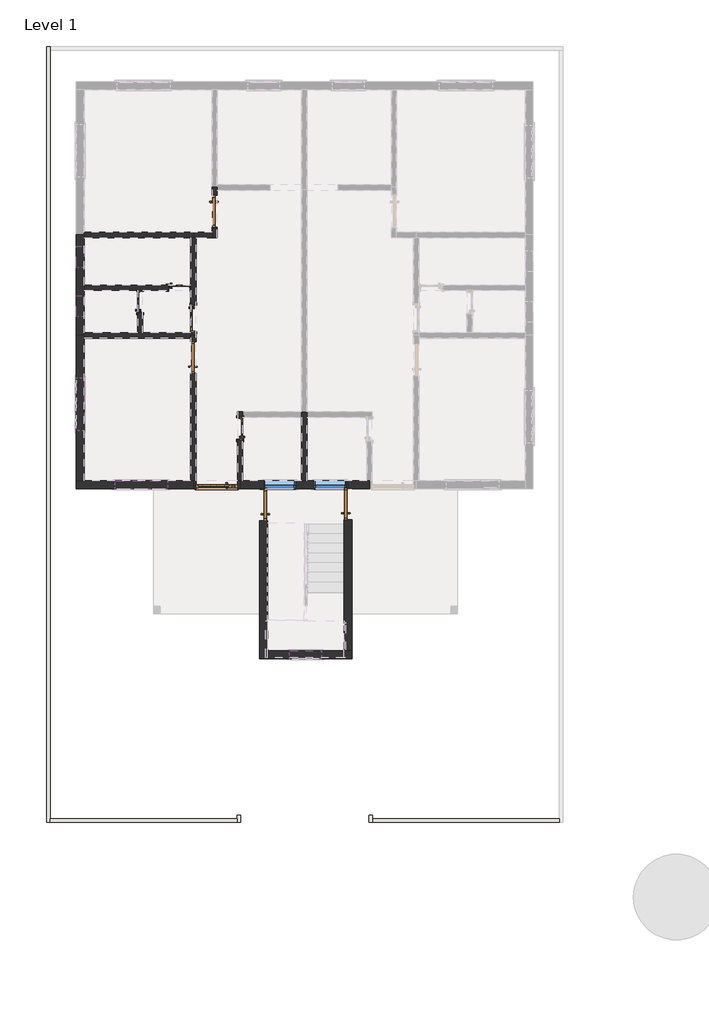
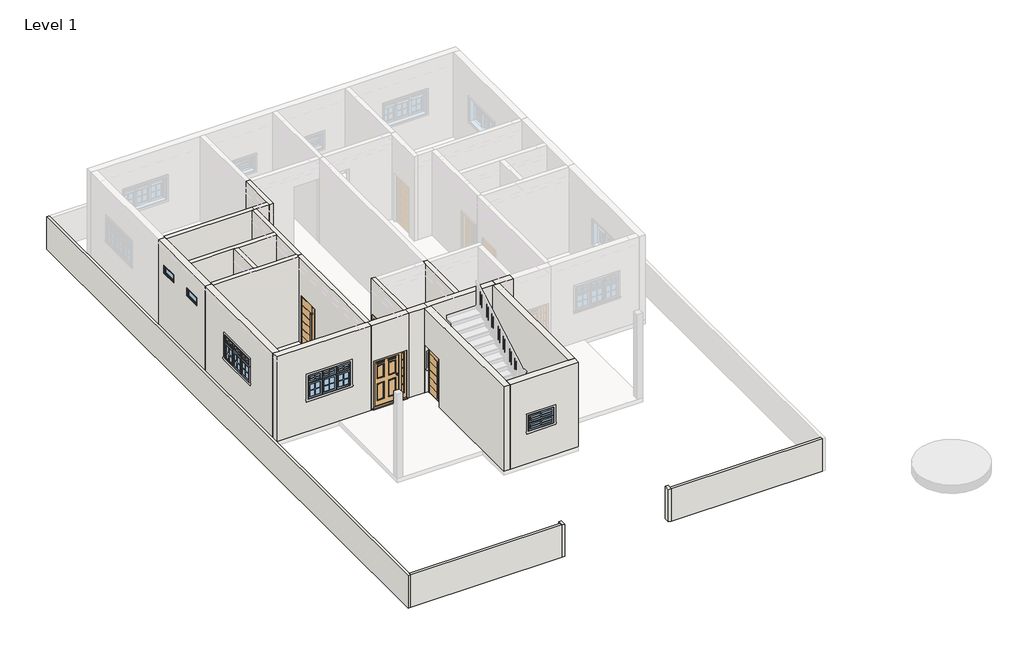
# One storey, part 1 of 4: 25 walls, 9 doors, 7 windows.
"""IFC4 building model written with IfcOpenShell, lengths in millimetres."""

from ifc_helpers import new_model, si_unit, frame, origin, place, context, project, spatial, polyline, outline, extrude, faceted_brep, transform, mapped, element, save
from components import door_3_ad1505b7, door_3_44036f4b, door_3_3562bf2b, door_3_abbf6f65, extsgl_w_side_panel_d749231e, m_door_interior_single_4_panel_wood_2_0346d007, m_door_interior_single_4_panel_wood_2_b7882c25, door_741bd24b, fixed_2_8c8825d0, m_window_awning_double_vertical_3_7e34f04a, m_window_casement_triple_awning_triple_5_96d5a87e

model = new_model("IFC4")

# Units and contexts
model_context = context("Model", 3, world=origin())
ifc_project = project(units=[si_unit("LENGTHUNIT", "METRE", prefix="MILLI")], contexts=[model_context])

# Site, building, storey
site = spatial("IfcSite", under=ifc_project)
building = spatial("IfcBuilding", under=site)
storey = spatial("IfcBuildingStorey", under=building, Name="Level 1", Elevation=0.0)

# Doors
placement = place(None, origin())
door_3_shape = door_3_ad1505b7(model_context)
element("IfcDoor", 1, ObjectType="3'", at=placement, inside=storey, context=model_context, shape_type="MappedRepresentation", body=[
    mapped(door_3_shape, transform((-10164.0299582, 11696.036641, 0.0), x_axis=(0.0, 1.0, 0.0), y_axis=(-1.0, 0.0, 0.0), z_axis=(0.0, 0.0, 1.0))),
])
door_3_2_shape = door_3_44036f4b(model_context)
element("IfcDoor", 2, ObjectType="3'", at=placement, inside=storey, context=model_context, shape_type="MappedRepresentation", body=[
    mapped(door_3_2_shape, transform((-9554.4299582, 15912.436641, 0.0), x_axis=(0.0, -1.0, 0.0), y_axis=(1.0, 0.0, 0.0), z_axis=(0.0, 0.0, 1.0))),
])
door_3_3_shape = door_3_3562bf2b(model_context)
element("IfcDoor", 3, ObjectType="3'", at=placement, inside=storey, context=model_context, shape_type="MappedRepresentation", body=[
    mapped(door_3_3_shape, transform((-8146.4581554, 7441.536641, 0.0), x_axis=(0.0, 1.0, 0.0), y_axis=(-1.0, 0.0, 0.0), z_axis=(0.0, 0.0, 1.0))),
])
door_3_4_shape = door_3_abbf6f65(model_context)
element("IfcDoor", 4, ObjectType="3'", at=placement, inside=storey, context=model_context, shape_type="MappedRepresentation", body=[
    mapped(door_3_4_shape, transform((-5708.0581554, 7466.936641, 0.0), x_axis=(0.0, 1.0, 0.0), y_axis=(-1.0, 0.0, 0.0), z_axis=(0.0, 0.0, 1.0))),
])
extsgl_w_side_panel_shape = extsgl_w_side_panel_d749231e(model_context)
element("IfcDoor", 5, ObjectType="ExtSgl w Side Panel", at=placement, inside=storey, context=model_context, shape_type="MappedRepresentation", body=[
    mapped(extsgl_w_side_panel_shape, transform((-9723.0299582, 8025.736641, 0.0), x_axis=(-1.0, 0.0, 0.0), y_axis=(0.0, -1.0, 0.0), z_axis=(0.0, 0.0, 1.0))),
])
m_door_interior_single_4_panel_wood_2_shape = m_door_interior_single_4_panel_wood_2_0346d007(model_context)
element("IfcDoor", 6, ObjectType="M_Door-Interior-Single-4_Panel-Wood : 2'", at=placement, inside=storey, context=model_context, shape_type="MappedRepresentation", body=[
    mapped(m_door_interior_single_4_panel_wood_2_shape, transform((-11703.9049582, 13296.236641, 0.0), x_axis=(0.0, 1.0, 0.0), y_axis=(-1.0, 0.0, 0.0), z_axis=(0.0, 0.0, 1.0))),
])
element("IfcDoor", 7, ObjectType="M_Door-Interior-Single-4_Panel-Wood : 2'", at=placement, inside=storey, context=model_context, shape_type="MappedRepresentation", body=[
    mapped(m_door_interior_single_4_panel_wood_2_shape, transform((-10570.4299582, 13705.811641, 0.0), x_axis=(1.0, 0.0, 0.0), y_axis=(0.0, 1.0, 0.0), z_axis=(0.0, 0.0, 1.0))),
])
m_door_interior_single_4_panel_wood_2_2_shape = m_door_interior_single_4_panel_wood_2_b7882c25(model_context)
element("IfcDoor", 8, ObjectType="M_Door-Interior-Single-4_Panel-Wood : 2'", at=placement, inside=storey, context=model_context, shape_type="MappedRepresentation", body=[
    mapped(m_door_interior_single_4_panel_wood_2_2_shape, transform((-8814.6549582, 9638.636641, 0.0), x_axis=(0.0, 1.0, 0.0), y_axis=(-1.0, 0.0, 0.0), z_axis=(0.0, 0.0, 1.0))),
])
door_shape = door_741bd24b(model_context)
element("IfcDoor", 9, ObjectType="M_Door-Interior-Single-6_Panel-Wood : 2'5\"", at=placement, inside=storey, context=model_context, shape_type="MappedRepresentation", body=[
    mapped(door_shape, transform((-10167.2049582, 12819.986641, 0.0), x_axis=(0.0, -1.0, 0.0), y_axis=(1.0, 0.0, 0.0), z_axis=(0.0, 0.0, 1.0))),
])

# Walls
element("IfcWall", 10, ObjectType="Generic - 4\"", at=placement, inside=storey, context=model_context, shape_type="Brep", body=[
    faceted_brep([(-14405.8299582, 20662.236641, -152.4), (-14405.8299582, -1715.163359, -152.4), (-14405.8299582, -1715.163359, 1066.8), (-14405.8299582, 20662.236641, 1066.8), (-14304.2299582, 20662.236641, -152.4), (-14304.2299582, 20662.236641, 1066.8), (-14304.2299582, 20560.636641, 1066.8), (-14304.2299582, -1613.563359, 1066.8), (-14304.2299582, -1715.163359, 1066.8), (-14304.2299582, -1715.163359, -152.4), (-14304.2299582, -1613.563359, -152.4), (-14304.2299582, 20560.636641, -152.4)], [[[0, 1, 2, 3]], [[4, 5, 6, 7, 8, 9, 10, 11]], [[1, 0, 4, 11, 10, 9]], [[3, 2, 8, 7, 6, 5]], [[2, 1, 9, 8]], [[0, 3, 5, 4]]]),
])
element("IfcWall", 11, ObjectType="Generic - 4\"", at=placement, inside=storey, context=model_context, shape_type="SweptSolid", body=[
    extrude(outline(polyline([(-8906.7299582, -1715.163359), (-14304.2299582, -1715.163359), (-14304.2299582, -1613.563359), (-8906.7299582, -1613.563359), (-8906.7299582, -1715.163359)])), frame((0.0, 0.0, -152.4), z_axis=(0.0, 0.0, 1.0), x_axis=(1.0, 0.0, 0.0)), (0.0, 0.0, 1.0), 1219.2),
])
element("IfcWall", 12, ObjectType="Generic - 4\"", at=placement, inside=storey, context=model_context, shape_type="Brep", body=[
    faceted_brep([(-8906.7299582, -1511.963359, -152.4), (-8906.7299582, -1613.563359, -152.4), (-8906.7299582, -1715.163359, -152.4), (-8906.7299582, -1715.163359, 1066.8), (-8906.7299582, -1613.563359, 1066.8), (-8906.7299582, -1511.963359, 1066.8), (-8805.1299582, -1511.963359, -152.4), (-8805.1299582, -1511.963359, 1066.8), (-8805.1299582, -1715.163359, 1066.8), (-8805.1299582, -1715.163359, -152.4)], [[[0, 1, 2, 3, 4, 5]], [[6, 7, 8, 9]], [[2, 1, 0, 6, 9]], [[5, 4, 3, 8, 7]], [[0, 5, 7, 6]], [[3, 2, 9, 8]]]),
])
element("IfcWall", 13, ObjectType="Generic - 4\"", at=placement, inside=storey, context=model_context, shape_type="SweptSolid", body=[
    extrude(outline(polyline([(-4995.1299582, -1613.563359), (402.3700418, -1613.563359), (402.3700418, -1715.163359), (-4995.1299582, -1715.163359), (-4995.1299582, -1613.563359)])), frame((0.0, 0.0, -152.4), z_axis=(0.0, 0.0, 1.0), x_axis=(1.0, 0.0, 0.0)), (0.0, 0.0, 1.0), 1219.2),
])
element("IfcWall", 14, ObjectType="Generic - 4\"", at=placement, inside=storey, context=model_context, shape_type="Brep", body=[
    faceted_brep([(-4995.1299582, -1715.163359, -152.4), (-4995.1299582, -1613.563359, -152.4), (-4995.1299582, -1511.963359, -152.4), (-4995.1299582, -1511.963359, 1066.8), (-4995.1299582, -1613.563359, 1066.8), (-4995.1299582, -1715.163359, 1066.8), (-5096.7299582, -1715.163359, -152.4), (-5096.7299582, -1715.163359, 1066.8), (-5096.7299582, -1511.963359, 1066.8), (-5096.7299582, -1511.963359, -152.4)], [[[0, 1, 2, 3, 4, 5]], [[6, 7, 8, 9]], [[2, 1, 0, 6, 9]], [[3, 2, 9, 8]], [[5, 4, 3, 8, 7]], [[0, 5, 7, 6]]]),
])
element("IfcWall", 15, ObjectType="Generic - 6\"", at=placement, inside=storey, context=model_context, shape_type="Brep", body=[
    faceted_brep([(-9630.6299582, 15302.836641, 0.0), (-10164.0299582, 15302.836641, 0.0), (-10164.0299582, 15302.836641, 3200.4), (-9630.6299582, 15302.836641, 3200.4), (-9630.6299582, 15150.436641, 0.0), (-9630.6299582, 15150.436641, 3200.4), (-10087.8299582, 15150.436641, 3200.4), (-10164.0299582, 15150.436641, 3200.4), (-10164.0299582, 15150.436641, 0.0), (-10087.8299582, 15150.436641, 0.0)], [[[0, 1, 2, 3]], [[4, 5, 6, 7, 8, 9]], [[1, 0, 4, 9, 8]], [[2, 1, 8, 7]], [[3, 2, 7, 6, 5]], [[0, 3, 5, 4]]]),
])
element("IfcWall", 16, ObjectType="Generic - 6\"", at=placement, inside=storey, context=model_context, shape_type="Brep", body=[
    faceted_brep([(-10240.2299582, 12331.036641, 0.0), (-10240.2299582, 12331.036641, 3200.4), (-10240.2299582, 12407.236641, 3200.4), (-10240.2299582, 13626.436641, 3200.4), (-10240.2299582, 13778.836641, 3200.4), (-10240.2299582, 15150.436641, 3200.4), (-10240.2299582, 15150.436641, 0.0), (-10240.2299582, 13778.836641, 0.0), (-10240.2299582, 13626.436641, 0.0), (-10240.2299582, 13219.986641, 0.0), (-10240.2299582, 13219.986641, 1853.8), (-10240.2299582, 12419.986641, 1853.8), (-10240.2299582, 12419.986641, 0.0), (-10240.2299582, 12407.236641, 0.0), (-10087.8299582, 12331.036641, 3200.4), (-10087.8299582, 12331.036641, 0.0), (-10087.8299582, 12419.986641, 0.0), (-10087.8299582, 12419.986641, 1853.8), (-10087.8299582, 13219.986641, 1853.8), (-10087.8299582, 13219.986641, 0.0), (-10087.8299582, 15150.436641, 0.0), (-10087.8299582, 15150.436641, 3200.4), (-10164.0299582, 15150.436641, 0.0), (-10164.0299582, 15150.436641, 3200.4)], [[[0, 1, 2, 3, 4, 5, 6, 7, 8, 9, 10, 11, 12, 13]], [[14, 15, 16, 17, 18, 19, 20, 21]], [[6, 22, 20, 19, 9, 8, 7]], [[15, 0, 13, 12, 16]], [[1, 0, 15, 14]], [[5, 4, 3, 2, 1, 14, 21, 23]], [[6, 5, 23, 21, 20, 22]], [[11, 17, 16, 12]], [[17, 11, 10, 18]], [[18, 10, 9, 19]]]),
])
element("IfcWall", 17, ObjectType="Generic - 6\"", at=placement, inside=storey, context=model_context, shape_type="Brep", body=[
    faceted_brep([(-10240.2299582, 12407.236641, 0.0), (-11624.5299582, 12407.236641, 0.0), (-11776.9299582, 12407.236641, 0.0), (-13313.6299582, 12407.236641, 0.0), (-13313.6299582, 12407.236641, 3200.4), (-11776.9299582, 12407.236641, 3200.4), (-11624.5299582, 12407.236641, 3200.4), (-10240.2299582, 12407.236641, 3200.4), (-10240.2299582, 12254.836641, 0.0), (-10240.2299582, 12254.836641, 3200.4), (-13313.6299582, 12254.836641, 3200.4), (-13313.6299582, 12254.836641, 0.0), (-10240.2299582, 12331.036641, 0.0), (-13313.6299582, 12331.036641, 0.0), (-13313.6299582, 12331.036641, 3200.4), (-10240.2299582, 12331.036641, 3200.4)], [[[0, 1, 2, 3, 4, 5, 6, 7]], [[8, 9, 10, 11]], [[3, 2, 1, 0, 12, 8, 11, 13]], [[7, 6, 5, 4, 14, 10, 9, 15]], [[4, 3, 13, 11, 10, 14]], [[0, 7, 15, 9, 8, 12]]]),
])
element("IfcWall", 18, ObjectType="Generic - 6\"", at=placement, inside=storey, context=model_context, shape_type="SweptSolid", body=[
    extrude(outline(polyline([(12407.236641, 3200.4), (13626.436641, 3200.4), (13626.436641, 0.0), (13626.036641, 0.0), (13626.036641, 1853.8), (12966.436641, 1853.8), (12966.436641, 0.0), (12407.236641, 0.0), (12407.236641, 3200.4)])), frame((-11776.9299582, 0.0, 0.0), z_axis=(1.0, 0.0, 0.0), x_axis=(0.0, 1.0, 0.0)), (0.0, 0.0, 1.0), 152.4),
])
element("IfcWall", 19, ObjectType="Generic - 6\"", at=placement, inside=storey, context=model_context, shape_type="Brep", body=[
    faceted_brep([(-10240.2299582, 13626.436641, 3200.4), (-11624.5299582, 13626.436641, 3200.4), (-11776.9299582, 13626.436641, 3200.4), (-13313.6299582, 13626.436641, 3200.4), (-13313.6299582, 13626.436641, 0.0), (-11776.9299582, 13626.436641, 0.0), (-11624.5299582, 13626.436641, 0.0), (-10900.2299582, 13626.436641, 0.0), (-10900.2299582, 13626.436641, 1853.8), (-10240.6299582, 13626.436641, 1853.8), (-10240.6299582, 13626.436641, 0.0), (-10240.2299582, 13626.436641, 0.0), (-13313.6299582, 13778.836641, 3200.4), (-10240.2299582, 13778.836641, 3200.4), (-10240.2299582, 13778.836641, 0.0), (-10240.6299582, 13778.836641, 0.0), (-10240.6299582, 13778.836641, 1853.8), (-10900.2299582, 13778.836641, 1853.8), (-10900.2299582, 13778.836641, 0.0), (-13313.6299582, 13778.836641, 0.0)], [[[0, 1, 2, 3, 4, 5, 6, 7, 8, 9, 10, 11]], [[12, 13, 14, 15, 16, 17, 18, 19]], [[4, 19, 18, 7, 6, 5]], [[14, 11, 10, 15]], [[3, 2, 1, 0, 13, 12]], [[4, 3, 12, 19]], [[0, 11, 14, 13]], [[9, 16, 15, 10]], [[16, 9, 8, 17]], [[17, 8, 7, 18]]]),
])
element("IfcWall", 20, ObjectType="Generic - 6\"", at=placement, inside=storey, context=model_context, shape_type="Brep", body=[
    faceted_brep([(-8741.6299582, 10121.236641, 3200.4), (-8741.6299582, 9968.836641, 3200.4), (-8741.6299582, 8140.036641, 3200.4), (-8741.6299582, 8140.036641, 0.0), (-8741.6299582, 9308.836641, 0.0), (-8741.6299582, 9308.836641, 1853.8), (-8741.6299582, 9968.436641, 1853.8), (-8741.6299582, 9968.436641, 0.0), (-8741.6299582, 9968.836641, 0.0), (-8741.6299582, 10121.236641, 0.0), (-8894.0299582, 8140.036641, 3200.4), (-8894.0299582, 10121.236641, 3200.4), (-8894.0299582, 10121.236641, 0.0), (-8894.0299582, 9968.436641, 0.0), (-8894.0299582, 9968.436641, 1853.8), (-8894.0299582, 9308.836641, 1853.8), (-8894.0299582, 9308.836641, 0.0), (-8894.0299582, 8140.036641, 0.0), (-8817.8299582, 8140.036641, 0.0), (-8817.8299582, 8140.036641, 3200.4)], [[[0, 1, 2, 3, 4, 5, 6, 7, 8, 9]], [[10, 11, 12, 13, 14, 15, 16, 17]], [[12, 9, 8, 7, 13]], [[3, 18, 17, 16, 4]], [[2, 1, 0, 11, 10, 19]], [[3, 2, 19, 10, 17, 18]], [[0, 9, 12, 11]], [[6, 14, 13, 7]], [[14, 6, 5, 15]], [[15, 5, 4, 16]]]),
])
element("IfcWall", 21, ObjectType="Generic - 6\"", at=placement, inside=storey, context=model_context, shape_type="Brep", body=[
    faceted_brep([(-9630.6299582, 15150.436641, 3200.4), (-9630.6299582, 15302.836641, 3200.4), (-9630.6299582, 16598.236641, 3200.4), (-9630.6299582, 16598.236641, 0.0), (-9630.6299582, 16369.636641, 0.0), (-9630.6299582, 16369.636641, 1828.8), (-9630.6299582, 15455.236641, 1828.8), (-9630.6299582, 15455.236641, 0.0), (-9630.6299582, 15302.836641, 0.0), (-9630.6299582, 15150.436641, 0.0), (-9478.2299582, 16598.236641, 3200.4), (-9478.2299582, 16522.036641, 3200.4), (-9478.2299582, 15150.436641, 3200.4), (-9478.2299582, 15150.436641, 0.0), (-9478.2299582, 15455.236641, 0.0), (-9478.2299582, 15455.236641, 1828.8), (-9478.2299582, 16369.636641, 1828.8), (-9478.2299582, 16369.636641, 0.0), (-9478.2299582, 16522.036641, 0.0), (-9478.2299582, 16598.236641, 0.0), (-9610.6299582, 15455.236641, 0.0), (-9610.6299582, 15440.236641, 0.0), (-9533.6299582, 15440.236641, 0.0), (-9533.6299582, 15455.236641, 0.0), (-9533.6299582, 16369.636641, 0.0), (-9533.6299582, 16384.636641, 0.0), (-9610.6299582, 16384.636641, 0.0), (-9610.6299582, 16369.636641, 0.0), (-9610.6299582, 16369.636641, 1828.8), (-9610.6299582, 15455.236641, 1828.8), (-9533.6299582, 15455.236641, 1828.8), (-9533.6299582, 16369.636641, 1828.8), (-9610.6299582, 16384.636641, 1843.8), (-9533.6299582, 16384.636641, 1843.8), (-9533.6299582, 15440.236641, 1843.8), (-9610.6299582, 15440.236641, 1843.8)], [[[0, 1, 2, 3, 4, 5, 6, 7, 8, 9]], [[10, 11, 12, 13, 14, 15, 16, 17, 18, 19]], [[13, 9, 8, 7, 20, 21, 22, 23, 14]], [[3, 19, 18, 17, 24, 25, 26, 27, 4]], [[2, 1, 0, 12, 11, 10]], [[3, 2, 10, 19]], [[0, 9, 13, 12]], [[5, 28, 29, 6]], [[15, 30, 31, 16]], [[30, 15, 14, 23]], [[6, 29, 20, 7]], [[16, 31, 24, 17]], [[28, 5, 4, 27]], [[32, 33, 34, 35]], [[35, 34, 22, 21]], [[31, 30, 23, 22, 34, 33, 25, 24]], [[33, 32, 26, 25]], [[29, 28, 27, 26, 32, 35, 21, 20]]]),
])
element("IfcWall", 22, ObjectType="Generic - 6\"", at=placement, inside=storey, context=model_context, shape_type="Brep", body=[
    faceted_brep([(-7039.8299582, 10108.536641, 0.0), (-7039.8299582, 9968.836641, 0.0), (-7039.8299582, 8140.036641, 0.0), (-7039.8299582, 8140.036641, 3200.4), (-7039.8299582, 9968.836641, 3200.4), (-7039.8299582, 10108.536641, 3200.4), (-6887.4299582, 10108.536641, 0.0), (-6887.4299582, 10108.536641, 3200.4), (-6887.4299582, 9968.836641, 3200.4), (-6887.4299582, 8140.036641, 3200.4), (-6887.4299582, 8140.036641, 0.0), (-6887.4299582, 9968.836641, 0.0)], [[[0, 1, 2, 3, 4, 5]], [[6, 7, 8, 9, 10, 11]], [[2, 1, 0, 6, 11, 10]], [[5, 4, 3, 9, 8, 7]], [[0, 5, 7, 6]], [[3, 2, 10, 9]]]),
])
element("IfcWall", 23, ObjectType="Generic - 6\"", at=placement, inside=storey, context=model_context, shape_type="Brep", body=[
    faceted_brep([(-10240.2299582, 8140.036641, 3200.4), (-10240.2299582, 12254.836641, 3200.4), (-10240.2299582, 12331.036641, 3200.4), (-10240.2299582, 12331.036641, 0.0), (-10240.2299582, 12254.836641, 0.0), (-10240.2299582, 12153.236641, 0.0), (-10240.2299582, 12153.236641, 1828.8), (-10240.2299582, 11238.836641, 1828.8), (-10240.2299582, 11238.836641, 0.0), (-10240.2299582, 8140.036641, 0.0), (-10087.8299582, 12331.036641, 3200.4), (-10087.8299582, 8140.036641, 3200.4), (-10087.8299582, 8140.036641, 1828.8), (-10087.8299582, 8140.036641, 0.0), (-10087.8299582, 11238.836641, 0.0), (-10087.8299582, 11238.836641, 1828.8), (-10087.8299582, 12153.236641, 1828.8), (-10087.8299582, 12153.236641, 0.0), (-10087.8299582, 12331.036641, 0.0), (-10164.0299582, 8140.036641, 0.0), (-10220.2299582, 11238.836641, 0.0), (-10220.2299582, 11223.836641, 0.0), (-10143.2299582, 11223.836641, 0.0), (-10143.2299582, 11238.836641, 0.0), (-10143.2299582, 12153.236641, 0.0), (-10143.2299582, 12168.236641, 0.0), (-10220.2299582, 12168.236641, 0.0), (-10220.2299582, 12153.236641, 0.0), (-10164.0299582, 8140.036641, 3200.4), (-10143.2299582, 11238.836641, 1828.8), (-10143.2299582, 12153.236641, 1828.8), (-10220.2299582, 12153.236641, 1828.8), (-10220.2299582, 11238.836641, 1828.8), (-10220.2299582, 11223.836641, 1843.8), (-10220.2299582, 12168.236641, 1843.8), (-10143.2299582, 12168.236641, 1843.8), (-10143.2299582, 11223.836641, 1843.8)], [[[0, 1, 2, 3, 4, 5, 6, 7, 8, 9]], [[10, 11, 12, 13, 14, 15, 16, 17, 18]], [[13, 19, 9, 8, 20, 21, 22, 23, 14]], [[3, 18, 17, 24, 25, 26, 27, 5, 4]], [[2, 1, 0, 28, 11, 10]], [[3, 2, 10, 18]], [[0, 9, 19, 13, 12, 11, 28]], [[15, 29, 30, 16]], [[6, 31, 32, 7]], [[16, 30, 24, 17]], [[31, 6, 5, 27]], [[29, 15, 14, 23]], [[7, 32, 20, 8]], [[33, 34, 35, 36]], [[35, 34, 26, 25]], [[30, 29, 23, 22, 36, 35, 25, 24]], [[33, 36, 22, 21]], [[32, 31, 27, 26, 34, 33, 21, 20]]]),
])
element("IfcWall", 24, ObjectType="Generic - 6\"", at=placement, inside=storey, context=model_context, shape_type="Brep", body=[
    faceted_brep([(-10164.0299582, 15302.836641, 0.0), (-13313.6299582, 15302.836641, 0.0), (-13313.6299582, 15302.836641, 3200.4), (-10164.0299582, 15302.836641, 3200.4), (-10164.0299582, 15150.436641, 0.0), (-10164.0299582, 15150.436641, 3200.4), (-10240.2299582, 15150.436641, 3200.4), (-13313.6299582, 15150.436641, 3200.4), (-13313.6299582, 15150.436641, 0.0), (-10240.2299582, 15150.436641, 0.0), (-13313.6299582, 15226.636641, 0.0), (-13313.6299582, 15226.636641, 3200.4)], [[[0, 1, 2, 3]], [[4, 5, 6, 7, 8, 9]], [[1, 0, 4, 9, 8, 10]], [[3, 2, 11, 7, 6, 5]], [[0, 3, 5, 4]], [[2, 1, 10, 8, 7, 11]]]),
])
element("IfcWall", 25, ObjectType="Generic - 9\"", at=placement, inside=storey, context=model_context, shape_type="Brep", body=[
    faceted_brep([(-13313.6299582, 8140.036641, 0.0), (-13313.6299582, 12254.836641, 0.0), (-13313.6299582, 12331.036641, 0.0), (-13313.6299582, 12331.036641, 3200.4), (-13313.6299582, 12254.836641, 3200.4), (-13313.6299582, 8140.036641, 3200.4), (-13313.6299582, 11102.311641, 2119.2), (-13313.6299582, 11102.311641, 1219.2), (-13313.6299582, 9578.311641, 1219.2), (-13313.6299582, 9578.311641, 2119.2), (-13542.2299582, 8140.036641, 0.0), (-13542.2299582, 8140.036641, 3200.4), (-13542.2299582, 12331.036641, 3200.4), (-13542.2299582, 12331.036641, 0.0), (-13542.2299582, 11102.311641, 2119.2), (-13542.2299582, 9578.311641, 2119.2), (-13542.2299582, 9578.311641, 1219.2), (-13542.2299582, 11102.311641, 1219.2)], [[[0, 1, 2, 3, 4, 5], [6, 7, 8, 9]], [[10, 11, 12, 13], [14, 15, 16, 17]], [[2, 1, 0, 10, 13]], [[3, 2, 13, 12]], [[5, 4, 3, 12, 11]], [[0, 5, 11, 10]], [[7, 6, 14, 17]], [[8, 7, 17, 16]], [[9, 8, 16, 15]], [[6, 9, 15, 14]]]),
])
element("IfcWall", 26, ObjectType="Generic - 9\"", at=placement, inside=storey, context=model_context, shape_type="Brep", body=[
    faceted_brep([(-8032.1581554, 7911.436641, 3200.4), (-8032.1581554, 3237.836641, 3200.4), (-8032.1581554, 3009.236641, 3200.4), (-8032.1581554, 3009.236641, 0.0), (-8032.1581554, 3237.836641, 0.0), (-8032.1581554, 6984.336641, 0.0), (-8032.1581554, 6984.336641, 1828.8), (-8032.1581554, 7898.736641, 1828.8), (-8032.1581554, 7898.736641, 0.0), (-8032.1581554, 7911.436641, 0.0), (-8260.7581554, 3009.236641, 3200.4), (-8260.7581554, 7911.436641, 3200.4), (-8260.7581554, 7911.436641, 0.0), (-8260.7581554, 7898.736641, 0.0), (-8260.7581554, 7898.736641, 1828.8), (-8260.7581554, 6984.336641, 1828.8), (-8260.7581554, 6984.336641, 0.0), (-8260.7581554, 3009.236641, 0.0), (-8129.1581554, 6984.336641, 0.0), (-8129.1581554, 6969.336641, 0.0), (-8052.1581554, 6969.336641, 0.0), (-8052.1581554, 6984.336641, 0.0), (-8052.1581554, 7898.736641, 0.0), (-8052.1581554, 7911.436641, 0.0), (-8146.4581554, 7911.436641, 0.0), (-8129.1581554, 7911.436641, 0.0), (-8129.1581554, 7898.736641, 0.0), (-8146.4581554, 7911.436641, 3200.4), (-8052.1581554, 7911.436641, 1843.8), (-8129.1581554, 7911.436641, 1843.8), (-8052.1581554, 6984.336641, 1828.8), (-8052.1581554, 7898.736641, 1828.8), (-8129.1581554, 7898.736641, 1828.8), (-8129.1581554, 6984.336641, 1828.8), (-8052.1581554, 6969.336641, 1843.8), (-8129.1581554, 6969.336641, 1843.8)], [[[0, 1, 2, 3, 4, 5, 6, 7, 8, 9]], [[10, 11, 12, 13, 14, 15, 16, 17]], [[3, 17, 16, 18, 19, 20, 21, 5, 4]], [[9, 8, 22, 23]], [[13, 12, 24, 25, 26]], [[2, 1, 0, 27, 11, 10]], [[0, 9, 23, 28, 29, 25, 24, 12, 11, 27]], [[3, 2, 10, 17]], [[6, 30, 31, 7]], [[14, 32, 33, 15]], [[7, 31, 22, 8]], [[32, 14, 13, 26]], [[30, 6, 5, 21]], [[15, 33, 18, 16]], [[34, 35, 29, 28]], [[33, 32, 26, 25, 29, 35, 19, 18]], [[35, 34, 20, 19]], [[31, 30, 21, 20, 34, 28, 23, 22]]]),
])
element("IfcWall", 27, ObjectType="Generic - 9\"", at=placement, inside=storey, context=model_context, shape_type="Brep", body=[
    faceted_brep([(-8032.1581554, 3009.236641, 0.0), (-5593.7581554, 3009.236641, 0.0), (-5593.7581554, 3009.236641, 3200.4), (-8032.1581554, 3009.236641, 3200.4), (-7384.4581554, 3009.236641, 1819.2), (-6470.0581554, 3009.236641, 1819.2), (-6470.0581554, 3009.236641, 1219.2), (-7384.4581554, 3009.236641, 1219.2), (-8032.1581554, 3237.836641, 0.0), (-8032.1581554, 3237.836641, 3200.4), (-5822.3581554, 3237.836641, 3200.4), (-5593.7581554, 3237.836641, 3200.4), (-5593.7581554, 3237.836641, 0.0), (-5822.3581554, 3237.836641, 0.0), (-7384.4581554, 3237.836641, 1819.2), (-7384.4581554, 3237.836641, 1219.2), (-6470.0581554, 3237.836641, 1219.2), (-6470.0581554, 3237.836641, 1819.2)], [[[0, 1, 2, 3], [4, 5, 6, 7]], [[8, 9, 10, 11, 12, 13], [14, 15, 16, 17]], [[1, 0, 8, 13, 12]], [[3, 2, 11, 10, 9]], [[0, 3, 9, 8]], [[2, 1, 12, 11]], [[15, 14, 4, 7]], [[16, 15, 7, 6]], [[17, 16, 6, 5]], [[14, 17, 5, 4]]]),
])
element("IfcWall", 28, ObjectType="Generic - 9\"", at=placement, inside=storey, context=model_context, shape_type="Brep", body=[
    faceted_brep([(-5593.7581554, 7911.436641, 3200.4), (-5593.7581554, 3237.836641, 3200.4), (-5593.7581554, 3237.836641, 0.0), (-5593.7581554, 7009.736641, 0.0), (-5593.7581554, 7009.736641, 1828.8), (-5593.7581554, 7911.436641, 1828.8), (-5822.3581554, 3237.836641, 3200.4), (-5822.3581554, 7911.436641, 3200.4), (-5822.3581554, 7911.436641, 1828.8), (-5822.3581554, 7009.736641, 1828.8), (-5822.3581554, 7009.736641, 0.0), (-5822.3581554, 3237.836641, 0.0), (-5802.3581554, 7009.736641, 0.0), (-5802.3581554, 6994.736641, 0.0), (-5725.3581554, 6994.736641, 0.0), (-5725.3581554, 7009.736641, 0.0), (-5708.0581554, 7911.436641, 3200.4), (-5708.0581554, 7911.436641, 1828.8), (-5725.3581554, 7911.436641, 1828.8), (-5725.3581554, 7911.436641, 1843.8), (-5802.3581554, 7911.436641, 1843.8), (-5802.3581554, 7911.436641, 1828.8), (-5802.3581554, 7009.736641, 1828.8), (-5725.3581554, 7009.736641, 1828.8), (-5725.3581554, 6994.736641, 1843.8), (-5802.3581554, 6994.736641, 1843.8)], [[[0, 1, 2, 3, 4, 5]], [[6, 7, 8, 9, 10, 11]], [[2, 11, 10, 12, 13, 14, 15, 3]], [[1, 0, 16, 7, 6]], [[2, 1, 6, 11]], [[7, 16, 0, 5, 17, 18, 19, 20, 21, 8]], [[22, 9, 8, 21]], [[4, 23, 18, 17, 5]], [[9, 22, 12, 10]], [[23, 4, 3, 15]], [[24, 25, 20, 19]], [[23, 15, 14, 24, 19, 18]], [[25, 24, 14, 13]], [[12, 22, 21, 20, 25, 13]]]),
])
element("IfcWall", 29, ObjectType="Generic - 9\"", at=placement, inside=storey, context=model_context, shape_type="Brep", body=[
    faceted_brep([(-5084.0299582, 8140.036641, 0.0), (-5160.2299582, 8140.036641, 0.0), (-5708.0581554, 8140.036641, 0.0), (-5708.0581554, 8140.036641, 3200.4), (-5160.2299582, 8140.036641, 3200.4), (-5084.0299582, 8140.036641, 3200.4), (-5084.0299582, 7911.436641, 3200.4), (-5593.7581554, 7911.436641, 3200.4), (-5708.0581554, 7911.436641, 3200.4), (-5708.0581554, 7911.436641, 1828.8), (-5593.7581554, 7911.436641, 1828.8), (-5593.7581554, 7911.436641, 0.0), (-5084.0299582, 7911.436641, 0.0), (-5593.7581554, 7924.136641, 0.0), (-5708.0581554, 7924.136641, 0.0), (-5708.0581554, 7924.136641, 1828.8), (-5593.7581554, 7924.136641, 1828.8)], [[[0, 1, 2, 3, 4, 5]], [[6, 7, 8, 9, 10, 11, 12]], [[2, 1, 0, 12, 11, 13, 14]], [[3, 2, 14, 15, 9, 8]], [[5, 4, 3, 8, 7, 6]], [[0, 5, 6, 12]], [[16, 13, 11, 10]], [[16, 10, 9, 15]], [[13, 16, 15, 14]]]),
])
element("IfcWall", 30, ObjectType="Generic - 9\"", at=placement, inside=storey, context=model_context, shape_type="Brep", body=[
    faceted_brep([(-10087.8299582, 8140.036641, 1828.8), (-10087.8299582, 8140.036641, 0.0), (-10164.0299582, 8140.036641, 0.0), (-10164.0299582, 8140.036641, 3200.4), (-10087.8299582, 8140.036641, 3200.4), (-8894.0299582, 8140.036641, 3200.4), (-8817.8299582, 8140.036641, 3200.4), (-8817.8299582, 8140.036641, 0.0), (-8894.0299582, 8140.036641, 0.0), (-8894.0299582, 8140.036641, 1828.8), (-10164.0299582, 7911.436641, 0.0), (-10087.8299582, 7911.436641, 0.0), (-10087.8299582, 7911.436641, 1828.8), (-8894.0299582, 7911.436641, 1828.8), (-8894.0299582, 7911.436641, 0.0), (-8817.8299582, 7911.436641, 0.0), (-8817.8299582, 7911.436641, 3200.4), (-10164.0299582, 7911.436641, 3200.4)], [[[0, 1, 2, 3, 4, 5, 6, 7, 8, 9]], [[10, 11, 12, 13, 14, 15, 16, 17]], [[8, 7, 15, 14]], [[2, 1, 11, 10]], [[3, 2, 10, 17]], [[6, 5, 4, 3, 17, 16]], [[7, 6, 16, 15]], [[13, 12, 0, 9]], [[12, 11, 1, 0]], [[14, 13, 9, 8]]]),
])
element("IfcWall", 31, ObjectType="Generic - 9\"", at=placement, inside=storey, context=model_context, shape_type="Brep", body=[
    faceted_brep([(-10164.0299582, 8140.036641, 0.0), (-10240.2299582, 8140.036641, 0.0), (-13313.6299582, 8140.036641, 0.0), (-13542.2299582, 8140.036641, 0.0), (-13542.2299582, 8140.036641, 3200.4), (-13313.6299582, 8140.036641, 3200.4), (-10240.2299582, 8140.036641, 3200.4), (-10164.0299582, 8140.036641, 3200.4), (-12430.9799582, 8140.036641, 2119.2), (-12430.9799582, 8140.036641, 1219.2), (-10906.9799582, 8140.036641, 1219.2), (-10906.9799582, 8140.036641, 2119.2), (-10164.0299582, 7911.436641, 0.0), (-10164.0299582, 7911.436641, 3200.4), (-13542.2299582, 7911.436641, 3200.4), (-13542.2299582, 7911.436641, 0.0), (-12430.9799582, 7911.436641, 2119.2), (-10906.9799582, 7911.436641, 2119.2), (-10906.9799582, 7911.436641, 1219.2), (-12430.9799582, 7911.436641, 1219.2)], [[[0, 1, 2, 3, 4, 5, 6, 7], [8, 9, 10, 11]], [[12, 13, 14, 15], [16, 17, 18, 19]], [[3, 2, 1, 0, 12, 15]], [[7, 6, 5, 4, 14, 13]], [[0, 7, 13, 12]], [[4, 3, 15, 14]], [[8, 11, 17, 16]], [[11, 10, 18, 17]], [[10, 9, 19, 18]], [[9, 8, 16, 19]]]),
])
element("IfcWall", 32, ObjectType="Generic - 9\"", at=placement, inside=storey, context=model_context, shape_type="Brep", body=[
    faceted_brep([(-13313.6299582, 12331.036641, 0.0), (-13313.6299582, 12407.236641, 0.0), (-13313.6299582, 13626.436641, 0.0), (-13313.6299582, 13778.836641, 0.0), (-13313.6299582, 15150.436641, 0.0), (-13313.6299582, 15226.636641, 0.0), (-13313.6299582, 15226.636641, 3200.4), (-13313.6299582, 15150.436641, 3200.4), (-13313.6299582, 13778.836641, 3200.4), (-13313.6299582, 13626.436641, 3200.4), (-13313.6299582, 12407.236641, 3200.4), (-13313.6299582, 12331.036641, 3200.4), (-13313.6299582, 13474.036641, 2438.4), (-13313.6299582, 13474.036641, 2133.6), (-13313.6299582, 12864.436641, 2133.6), (-13313.6299582, 12864.436641, 2438.4), (-13313.6299582, 14896.436641, 2438.4), (-13313.6299582, 14896.436641, 2133.6), (-13313.6299582, 14286.836641, 2133.6), (-13313.6299582, 14286.836641, 2438.4), (-13542.2299582, 12331.036641, 0.0), (-13542.2299582, 12331.036641, 3200.4), (-13542.2299582, 15226.636641, 3200.4), (-13542.2299582, 15226.636641, 0.0), (-13542.2299582, 13474.036641, 2438.4), (-13542.2299582, 12864.436641, 2438.4), (-13542.2299582, 12864.436641, 2133.6), (-13542.2299582, 13474.036641, 2133.6), (-13542.2299582, 14896.436641, 2438.4), (-13542.2299582, 14286.836641, 2438.4), (-13542.2299582, 14286.836641, 2133.6), (-13542.2299582, 14896.436641, 2133.6)], [[[0, 1, 2, 3, 4, 5, 6, 7, 8, 9, 10, 11], [12, 13, 14, 15], [16, 17, 18, 19]], [[20, 21, 22, 23], [24, 25, 26, 27], [28, 29, 30, 31]], [[5, 4, 3, 2, 1, 0, 20, 23]], [[6, 5, 23, 22]], [[11, 10, 9, 8, 7, 6, 22, 21]], [[0, 11, 21, 20]], [[12, 15, 25, 24]], [[15, 14, 26, 25]], [[14, 13, 27, 26]], [[13, 12, 24, 27]], [[16, 19, 29, 28]], [[19, 18, 30, 29]], [[18, 17, 31, 30]], [[17, 16, 28, 31]]]),
])
element("IfcWall", 33, ObjectType="Generic - 9\"", at=placement, inside=storey, context=model_context, shape_type="Brep", body=[
    faceted_brep([(-8146.4581554, 8140.036641, 0.0), (-8741.6299582, 8140.036641, 0.0), (-8817.8299582, 8140.036641, 0.0), (-8817.8299582, 8140.036641, 3200.4), (-8741.6299582, 8140.036641, 3200.4), (-8146.4581554, 8140.036641, 3200.4), (-8817.8299582, 7911.436641, 0.0), (-8260.7581554, 7911.436641, 0.0), (-8146.4581554, 7911.436641, 0.0), (-8146.4581554, 7911.436641, 3200.4), (-8260.7581554, 7911.436641, 3200.4), (-8817.8299582, 7911.436641, 3200.4)], [[[0, 1, 2, 3, 4, 5]], [[6, 7, 8, 9, 10, 11]], [[2, 1, 0, 8, 7, 6]], [[3, 2, 6, 11]], [[5, 4, 3, 11, 10, 9]], [[0, 5, 9, 8]]]),
])
element("IfcWall", 34, ObjectType="Generic - 9\"", at=placement, inside=storey, context=model_context, shape_type="Brep", body=[
    faceted_brep([(-5708.0581554, 8140.036641, 0.0), (-6887.4299582, 8140.036641, 0.0), (-7039.8299582, 8140.036641, 0.0), (-8146.4581554, 8140.036641, 0.0), (-8146.4581554, 8140.036641, 3200.4), (-7039.8299582, 8140.036641, 3200.4), (-6887.4299582, 8140.036641, 3200.4), (-5708.0581554, 8140.036641, 3200.4), (-8137.7269054, 8140.036641, 1500.0), (-8137.7269054, 8140.036641, 900.0), (-7223.3269054, 8140.036641, 900.0), (-7223.3269054, 8140.036641, 1500.0), (-6676.4331554, 8140.036641, 1500.0), (-6676.4331554, 8140.036641, 900.0), (-5762.0331554, 8140.036641, 900.0), (-5762.0331554, 8140.036641, 1500.0), (-8146.4581554, 7911.436641, 3200.4), (-8146.4581554, 7911.436641, 0.0), (-8129.1581554, 7911.436641, 0.0), (-8129.1581554, 7911.436641, 900.0), (-8137.7269054, 7911.436641, 900.0), (-8137.7269054, 7911.436641, 1500.0), (-8129.1581554, 7911.436641, 1500.0), (-8129.1581554, 7911.436641, 1843.8), (-8052.1581554, 7911.436641, 1843.8), (-8052.1581554, 7911.436641, 1500.0), (-7223.3269054, 7911.436641, 1500.0), (-7223.3269054, 7911.436641, 900.0), (-8052.1581554, 7911.436641, 900.0), (-8052.1581554, 7911.436641, 0.0), (-8032.1581554, 7911.436641, 0.0), (-5822.3581554, 7911.436641, 0.0), (-5822.3581554, 7911.436641, 900.0), (-6676.4331554, 7911.436641, 900.0), (-6676.4331554, 7911.436641, 1500.0), (-5822.3581554, 7911.436641, 1500.0), (-5822.3581554, 7911.436641, 1828.8), (-5802.3581554, 7911.436641, 1828.8), (-5802.3581554, 7911.436641, 1843.8), (-5725.3581554, 7911.436641, 1843.8), (-5725.3581554, 7911.436641, 1828.8), (-5708.0581554, 7911.436641, 1828.8), (-5708.0581554, 7911.436641, 3200.4), (-5822.3581554, 7911.436641, 3200.4), (-8032.1581554, 7911.436641, 3200.4), (-5708.0581554, 7924.136641, 0.0), (-5725.3581554, 7924.136641, 0.0), (-5725.3581554, 7939.136641, 0.0), (-5802.3581554, 7939.136641, 0.0), (-5802.3581554, 7924.136641, 0.0), (-5822.3581554, 7924.136641, 0.0), (-8052.1581554, 7913.736641, 0.0), (-8129.1581554, 7913.736641, 0.0), (-5708.0581554, 7924.136641, 1828.8), (-8129.1581554, 7913.736641, 900.0), (-8052.1581554, 7913.736641, 900.0), (-8052.1581554, 7913.736641, 1500.0), (-8129.1581554, 7913.736641, 1500.0), (-5822.3581554, 7924.136641, 900.0), (-5802.3581554, 7924.136641, 900.0), (-5802.3581554, 7939.136641, 900.0), (-5762.0331554, 7939.136641, 900.0), (-5762.0331554, 7939.136641, 1500.0), (-5802.3581554, 7939.136641, 1500.0), (-5802.3581554, 7924.136641, 1500.0), (-5822.3581554, 7924.136641, 1500.0), (-8129.1581554, 7913.736641, 1843.8), (-8052.1581554, 7913.736641, 1843.8), (-5822.3581554, 7924.136641, 1828.8), (-5802.3581554, 7924.136641, 1828.8), (-5725.3581554, 7924.136641, 1828.8), (-5802.3581554, 7939.136641, 1843.8), (-5725.3581554, 7939.136641, 1843.8)], [[[0, 1, 2, 3, 4, 5, 6, 7], [8, 9, 10, 11], [12, 13, 14, 15]], [[16, 17, 18, 19, 20, 21, 22, 23, 24, 25, 26, 27, 28, 29, 30, 31, 32, 33, 34, 35, 36, 37, 38, 39, 40, 41, 42, 43, 44]], [[3, 2, 1, 0, 45, 46, 47, 48, 49, 50, 31, 30, 29, 51, 52, 18, 17]], [[4, 3, 17, 16]], [[7, 6, 5, 4, 16, 44, 43, 42]], [[0, 7, 42, 41, 53, 45]], [[8, 21, 20, 9]], [[9, 20, 19, 54, 55, 28, 27, 10]], [[10, 27, 26, 11]], [[21, 8, 11, 26, 25, 56, 57, 22]], [[12, 34, 33, 13]], [[13, 33, 32, 58, 59, 60, 61, 14]], [[15, 14, 61, 62]], [[34, 12, 15, 62, 63, 64, 65, 35]], [[66, 67, 24, 23]], [[67, 66, 57, 56]], [[54, 52, 51, 55]], [[66, 23, 22, 57]], [[52, 54, 19, 18]], [[24, 67, 56, 25]], [[55, 51, 29, 28]], [[50, 58, 32, 31]], [[65, 68, 36, 35]], [[68, 69, 37, 36]], [[40, 70, 53, 41]], [[69, 68, 65, 64]], [[70, 46, 45, 53]], [[58, 50, 49, 59]], [[71, 72, 39, 38]], [[72, 71, 63, 62, 61, 60, 48, 47]], [[46, 70, 40, 39, 72, 47]], [[37, 69, 64, 63, 71, 38]], [[59, 49, 48, 60]]]),
])

# Windows
fixed_2_shape = fixed_2_8c8825d0(model_context)
element("IfcWindow", 35, ObjectType="Fixed : 2'", at=placement, inside=storey, context=model_context, shape_type="MappedRepresentation", body=[
    mapped(fixed_2_shape, transform((-13427.9299582, 13207.336641, 1219.2), x_axis=(0.0, 1.0, 0.0), y_axis=(-1.0, 0.0, 0.0), z_axis=(0.0, 0.0, 1.0))),
])
element("IfcWindow", 36, ObjectType="Fixed : 2'", at=placement, inside=storey, context=model_context, shape_type="MappedRepresentation", body=[
    mapped(fixed_2_shape, transform((-13427.9299582, 14629.736641, 1219.2), x_axis=(0.0, 1.0, 0.0), y_axis=(-1.0, 0.0, 0.0), z_axis=(0.0, 0.0, 1.0))),
])
m_window_awning_double_vertical_3_shape = m_window_awning_double_vertical_3_7e34f04a(model_context)
element("IfcWindow", 37, ObjectType="M_Window-Awning-Double-Vertical : 3'", at=placement, inside=storey, context=model_context, shape_type="MappedRepresentation", body=[
    mapped(m_window_awning_double_vertical_3_shape, transform((-7680.5269054, 8025.736641, 0.0), x_axis=(-1.0, 0.0, 0.0), y_axis=(0.0, -1.0, 0.0), z_axis=(0.0, 0.0, 1.0))),
])
element("IfcWindow", 38, ObjectType="M_Window-Awning-Double-Vertical : 3'", at=placement, inside=storey, context=model_context, shape_type="MappedRepresentation", body=[
    mapped(m_window_awning_double_vertical_3_shape, transform((-6219.2331554, 8025.736641, 0.0), x_axis=(-1.0, 0.0, 0.0), y_axis=(0.0, -1.0, 0.0), z_axis=(0.0, 0.0, 1.0))),
])
element("IfcWindow", 39, ObjectType="M_Window-Awning-Double-Vertical : 3'", at=placement, inside=storey, context=model_context, shape_type="MappedRepresentation", body=[
    mapped(m_window_awning_double_vertical_3_shape, transform((-6927.2581554, 3123.536641, 319.2), x_axis=(-1.0, 0.0, 0.0), y_axis=(0.0, -1.0, 0.0), z_axis=(0.0, 0.0, 1.0))),
])
m_window_casement_triple_awning_triple_5_shape = m_window_casement_triple_awning_triple_5_96d5a87e(model_context)
element("IfcWindow", 40, ObjectType="M_Window-Casement-Triple-Awning-Triple : 5'", at=placement, inside=storey, context=model_context, shape_type="MappedRepresentation", body=[
    mapped(m_window_casement_triple_awning_triple_5_shape, transform((-11668.9799582, 8025.736641, 319.2), x_axis=(-1.0, 0.0, 0.0), y_axis=(0.0, -1.0, 0.0), z_axis=(0.0, 0.0, 1.0))),
])
element("IfcWindow", 41, ObjectType="M_Window-Casement-Triple-Awning-Triple : 5'", at=placement, inside=storey, context=model_context, shape_type="MappedRepresentation", body=[
    mapped(m_window_casement_triple_awning_triple_5_shape, transform((-13427.9299582, 10340.311641, 319.2), x_axis=(0.0, 1.0, 0.0), y_axis=(-1.0, 0.0, 0.0), z_axis=(0.0, 0.0, 1.0))),
])

save(model, "model.ifc")

# Revit data of these elements
# Type "3'"
#   Type Mark = "9"
#   Water resistance = "up to Class E900, EN 12208:2001"
#   Uniclass2015Version = "v1.21"
#   Uniclass2015Reference = "Ss_25_30_20_30"
#   Uniclass2015Description = "Frame and door leaf system"
#   URL = "www.aluprof.com"
#   Type IFC Predefined Type = "USERDEFINED"
#   Right-hand / Left-hand door [instance default] = ""
#   Resistance to wind load = "up to Class C5/B5, EN 12210:2001"
#   Insert type = "ST"
#   Hardware [instance default] = ""
#   Product page = "https://aluprof.com/en/architects/offer/window-and-door-systems/panel-doors#visualisation"
#   Operation = "SinglePanelOutwardOpening"
#   Opening type = "Outward"
#   NBSReference = "25-50-20/125"
#   NBSDescription = "Frame and door leaf system"
#   Important = "The actual acceptable construction dimensions are dependent on the selection of profiles and hardware, glazing type, construction weight and the construction’s operating conditions. These should be determined by a suitably qualified person, and using ALUPROF’s calculation software"
#   IfcExportType = "USERDEFINED"
#   IfcExportAs = "IfcDoorType"
#   Handle type [instance default] = ""
#   Manufacturer = "ALUPROF SA"
#   Export Type to IFC As = "IfcDoorType"
#   Door sill type [instance default] = ""
#   Description = "External single-leaf panel door outward opening"
#   Model = "MB-86 ST Panel Door AD07"
#   Content of the recyclate in the material = "69.2%"
#   COBie.Type.WarrantyDurationParts = ""
#   COBie.Type.Name = ""
#   COBie.Type.Manufacturer = "ALUPROF SA"
#   COBie.Space.Name = ""
#   COBie.Floor.Name = ""
#   COBie.Facility.Name = ""
#   COBie.CreatedOn = ""
#   COBie.Component.WarrantyStartDate = ""
#   COBie.Component.Name = "MB-86 ST Panel Door AD07"
#   Burglar resistance = "RC2"
#   Air permeability = "up to Class 4, EN 12207:2001"
#   Width of the active leaf = 2' - 8.17717"
#   Placement in wall = 0' - 0.7874"
#   Thickness = 0' - 3.0315"
#   Height of the opening sash = 5' - 9.44094"
#   Handle Offset = 3' - 5.33858"
#   Rough Height = 6' - 2.40945"
#   Rough Width = 3' - 1.1811"
#   Height = 6' - 0"
#   Width = 3' - 0"
#   Construction depth = 0' - 3.0315"
#   Clear opening width = 2' - 3.94882"
#   Clear opening height = 5' - 8.47638"
#   Height of the array = 0' - 11.08136"
#   Schedule No. [instance default] = 1
#   Handrail [instance default] = yes
#   IsExternal = yes
#   Handle [instance default] = no
#   Door closer [instance default] = no
#   Function = 1
#   COBie.Type = yes
#   COBie = yes
#   Access control [instance default] = no
#   Panel = element 380416
#   Wall Closure = (empty or 0)
# Type "ExtSgl w Side Panel"
#   Type Mark = "14"
#   Operation = "SingleSwingRight"
#   Keynote = "L20"
#   Wrap Layers (Int) from Ext = 0' - 6.98819"
#   Wrap Layers (Ext) from Ext = 0' - 4.03543"
#   Thickness = 0' - 1.73228"
#   Stile Top of Lock rail = 3' - 3.37008"
#   Stile Top of Frieze Rail = 5' - 3.97638"
#   Stile Top Rail = 0' - 5.90551"
#   Stile Shutting = 0' - 4.92126"
#   Panelling Widths = 0' - 9.84252"
#   Stile Lock Rail = 0' - 6.88976"
#   Stile Intermediate/Frieze = 0' - 4.92126"
#   Stile Hanging = 0' - 4.92126"
#   Stile Bottom Rail = 0' - 6.88976"
#   Rough Width = 3' - 11"
#   Rough Height = 6' - 0"
#   O/A Frame Width = 0' - 2.51969"
#   Handle Z Distance = 3' - 3.37008"
#   Glazing Thickness = 0' - 0.94488"
#   Glazing Bar Thickness = 0' - 0.98425"
#   FrameWidth = 0' - 1.65354"
#   FrameOffset - External = 0' - 0.98425"
#   FrameDepth = 0' - 3.50394"
#   Door Panel Width = 2' - 11.70866"
#   Door Panel Thickness = 0' - 1.73228"
#   Door Panel Height = 5' - 7.66929"
#   Cill Thickness = 0' - 2.14567"
#   Cill Projection = 0' - 1.1811"
#   Handle X Distance = 0' - 2.95276"
#   Height = 6' - 0"
#   Structural Tolerance = 0' - 0.25591"
#   Tolerance = 0' - 0.11811"
#   Undercut = 0' - 0.15748"
#   Width = 3' - 11"
#   Cill Extension = 0' - 0.98425"
#   Cavity Closer Width = 0' - 1.9685"
#   Cavity Closer Offset from Ext = 0' - 4.03543"
#   Cavity Closer Depth = 0' - 3.34646"
#   Vis - SideLight Glazing Bars = yes
#   Vis - Ironmongery = yes
#   Vis - Cavity Closers = yes
#   Function = 1
#   Material Glass = Door - Glazing
#   Handle Style = element 390192
#   Material Door = Door - Panel
#   Material Ironmongery = Door - Handle
#   Wall Closure = (empty or 0)
# Type "M_Door-Interior-Single-4_Panel-Wood : 2'"
#   Type Mark = "13"
#   Assembly Code = "C1020300"
#   Analytic Construction = "Wooden"
#   Top Rail = 0' - 4.72441"
#   Thickness = 0' - 1.37795"
#   Thermal Resistance (R) = 2.5876 (h·ft²·°F)/BTU
#   Swing Angle [instance default] = 90.00°
#   Stiles = 0' - 4.72441"
#   Rough Width = 2' - 1.9685"
#   Rough Height = 6' - 0.98425"
#   Mullion = 0' - 4.52756"
#   Lock Rail = 0' - 7.87402"
#   Height = 6' - 0"
#   Width = 2' - 0"
#   Heat Transfer Coefficient (U) = 0.3865 BTU/(h·ft²·°F)
#   Bottom Rail = 0' - 9.05512"
#   Trim Material = Cherry
#   Panel Material = Cherry
#   Frame Material = Cherry
#   Door Handle Material = Aluminum
#   Visual Light Transmittance = 0
#   Solar Heat Gain Coefficient = 0
#   Wall Closure = (empty or 0)
#   Function = (empty or 0)
# Type "M_Door-Interior-Single-6_Panel-Wood : 2'5\""
#   Type Mark = "11"
#   Assembly Code = "C1020300"
#   Analytic Construction = "Wooden"
#   Top Rail = 0' - 4.72441"
#   Top Panel = 0' - 7.77559"
#   Thickness = 0' - 1.37795"
#   Thermal Resistance (R) = 2.5876 (h·ft²·°F)/BTU
#   Swing Angle [instance default] = 90.00°
#   Stiles = 0' - 4.72441"
#   Rough Width = 2' - 7.49606"
#   Rough Height = 6' - 0.98425"
#   Mullion = 0' - 4.52756"
#   Lock Rail = 0' - 7.87402"
#   Intermediate Rail = 0' - 4.52756"
#   Height = 6' - 0"
#   Width = 2' - 5.52756"
#   Heat Transfer Coefficient (U) = 0.3865 BTU/(h·ft²·°F)
#   Bottom Rail = 0' - 9.05512"
#   Trim Material = Cherry
#   Panel Material = Cherry
#   Frame Material = Cherry
#   Door Handle Material = Aluminum
#   Visual Light Transmittance = 0
#   Solar Heat Gain Coefficient = 0
#   Wall Closure = (empty or 0)
#   Function = (empty or 0)
# Type "Generic - 4\""
#   Assembly Code = "B2010"
#   Layers, outside or top first: 0' - 4" no material (function 1)
# Type "Generic - 6\""
#   Assembly Code = "B2010"
#   Layers, outside or top first: 0' - 6" no material (function 1)
# Type "Generic - 9\""
#   Assembly Code = "B2010"
#   Layers, outside or top first: 0' - 9" no material (function 1)
# Type "Fixed : 2'"
#   Type Mark = "23"
#   Construction Type Id = "GSP4R"
#   Assembly Code = "B2020100"
#   Analytic Construction = "1/8 in Pilkington single glazing"
#   Visual Light Transmittance = 0.9
#   Solar Heat Gain Coefficient = 0.78
#   Heat Transfer Coefficient (U) = 0.6496 BTU/(h·ft²·°F)
#   Height = 1' - 0"
#   Default Sill Height = 3' - 0"
#   Width = 2' - 0"
#   Window Inset = 0' - 0 3/4"
#   Define Thermal Properties by = 1
#   Glass Pane Material = Glass
#   Sash Material = Sash
#   Wall Closure = (empty or 0)
# Type "M_Window-Awning-Double-Vertical : 3'"
#   Type Mark = "22"
#   Fire Rating = "0.5h"
#   Assembly Code = "B2020100"
#   Analytic Construction = "Double glazing - domestic"
#   Window Inset [instance default] = 0' - 0"
#   Wall Thickness [instance default] = 0' - 5.90551"
#   Visual Light Transmittance = 0.81
#   Top Sash Height Ratio = 0.5
#   Top Sash Height = 0' - 11.81102"
#   Thermal Resistance (R) = 1.8146 (h·ft²·°F)/BTU
#   Solar Heat Gain Coefficient = 0.76
#   Rough Width = 3' - 0.59055"
#   Rough Height = 2' - 0.2126"
#   Interior Wall Closure [instance default] = 0' - 2.15551"
#   Height = 1' - 11.62205"
#   Heat Transfer Coefficient (U) = 0.5511 BTU/(h·ft²·°F)
#   Frame Extension [instance default] = 0' - 0 1/4"
#   Exterior Wall Closure [instance default] = 0' - 1 1/4"
#   Extension Jamb [instance default] = 0' - 2.15551"
#   Default Sill Height = 2' - 11.43307"
#   Width = 3' - 0"
#   Top Muntin Visibility = yes
#   Interior Trim Visibility [instance default] = yes
#   Exterior Trim Visibility [instance default] = yes
#   Extension Jamb Visibility [instance default] = yes
#   Bottom Muntin Visibility = yes
#   Muntin Pattern = M_Muntin Pattern_2x2 : M_Muntin Pattern_2x2
#   Interior Trim Material = Wood - Stained
#   Interior Trim = M_Trim-Window-Interior-Flat : Picture Frame
#   Interior Frame Material = Wood - Stained
#   Glass Panel Material = Glass
#   Exterior Trim Material = Clad - White
#   Exterior Trim = M_Trim-Window-Exterior-Flat : with Sill
#   Exterior Frame Material = Clad - White
#   Wall Closure = (empty or 0)
# Type "M_Window-Casement-Triple-Awning-Triple : 5'"
#   Type Mark = "19"
#   Fire Rating = "0.5h"
#   Assembly Code = "B2020100"
#   Analytic Construction = "Double glazing - domestic"
#   Window Inset [instance default] = 0' - 0"
#   Wall Thickness [instance default] = 0' - 5.90551"
#   One Third Width = 1' - 8"
#   Visual Light Transmittance = 0.81
#   Transom Height = 0' - 11.81102"
#   Thermal Resistance (R) = 1.8146 (h·ft²·°F)/BTU
#   Solar Heat Gain Coefficient = 0.76
#   Sash Width = 1' - 7.16667"
#   Rough Width = 5' - 0.59055"
#   Rough Height = 3' - 0.02362"
#   Open Window Height = 1' - 11.62205"
#   Frame Extension [instance default] = 0' - 0 1/4"
#   Interior Wall Closure [instance default] = 0' - 2.15551"
#   Height = 2' - 11.43307"
#   Heat Transfer Coefficient (U) = 0.5511 BTU/(h·ft²·°F)
#   Exterior Wall Closure [instance default] = 0' - 1 1/4"
#   Extension Jamb [instance default] = 0' - 2.15551"
#   Default Sill Height = 2' - 11.43307"
#   Width = 5' - 0"
#   Top Side Muntin Visibility = yes
#   Top Middle Muntin Visibility = yes
#   Bottom Side Muntin Visibility = yes
#   Bottom Middle Muntin Visibility = yes
#   Interior Trim Visibility [instance default] = yes
#   Exterior Trim Visibility [instance default] = yes
#   Extension Jamb Visibility [instance default] = yes
#   Muntin Pattern = M_Muntin Pattern_2x2 : M_Muntin Pattern_2x2
#   Interior Trim Material = Wood - Stained
#   Interior Trim = M_Trim-Window-Interior-Flat : Picture Frame
#   Interior Frame Material = Wood - Stained
#   Glass Panel Material = Glass
#   Exterior Trim Material = Clad - White
#   Exterior Trim = M_Trim-Window-Exterior-Flat : with Sill
#   Exterior Frame Material = Clad - White
#   Wall Closure = (empty or 0)
# Elements 1, 2, 3, 4 (IfcDoor, "3'")
#   Right-hand / Left-hand door = ""
#   Hardware = ""
#   Handle type = ""
#   Door sill type = ""
#   Schedule No. = 1
#   Handrail = yes
#   Handle = no
#   Door closer = no
#   Access control = no
#   Phase Created = New Construction
# Element 5 (IfcDoor, "ExtSgl w Side Panel")
#   Phase Created = New Construction
#   Materials on its faces: "Door - Panel", "Door - Handle", "Door - Glazing"
# Elements 6, 7, 8 (IfcDoor, "M_Door-Interior-Single-4_Panel-Wood : 2'")
#   Swing Angle = 90.00°
#   Phase Created = New Construction
#   Materials on its faces: "Cherry", "Aluminum"
# Element 9 (IfcDoor, "M_Door-Interior-Single-6_Panel-Wood : 2'5\"")
#   Swing Angle = 90.00°
#   Phase Created = New Construction
#   Materials on its faces: "Cherry", "Aluminum"
# Element 10 (IfcWall, "Generic - 4\"")
#   built-in parameter 1001111 = -0' - 6"
#   Top Offset = 0' - 0"
#   Base Offset = -0' - 6"
#   Unconnected Height = 4' - 0"
#   wall height = 4' - 0"
#   Phase Created = New Construction
#   Base Constraint = Level 1
#   Materials on its faces: "LVW1", "Default Wall"
# Elements 11, 12, 13, 14 (IfcWall, "Generic - 4\"")
#   built-in parameter 1001111 = -0' - 6"
#   Top Offset = 0' - 0"
#   Base Offset = -0' - 6"
#   Unconnected Height = 4' - 0"
#   wall height = 4' - 0"
#   Phase Created = New Construction
#   Base Constraint = Level 1
#   Materials on its faces: "Default Wall", "LVW1"
# Elements 15, 23 (IfcWall, "Generic - 6\"")
#   Top Offset = 0' - 0"
#   Base Offset = 0' - 0"
#   Unconnected Height = 10' - 6"
#   wall height = 10' - 6"
#   Phase Created = New Construction
#   Base Constraint = Level 1
#   Materials on its faces: "Default Wall", "BED ROOM WALL 2"
# Elements 16, 19, 22 (IfcWall, "Generic - 6\"")
#   Top Offset = 0' - 0"
#   Base Offset = 0' - 0"
#   Unconnected Height = 10' - 6"
#   wall height = 10' - 6"
#   Phase Created = New Construction
#   Base Constraint = Level 1
#   Materials on its faces: "Default Wall", "BAW1"
# Element 17 (IfcWall, "Generic - 6\"")
#   Top Offset = 0' - 0"
#   Base Offset = 0' - 0"
#   Unconnected Height = 10' - 6"
#   wall height = 10' - 6"
#   Phase Created = New Construction
#   Base Constraint = Level 1
#   Materials on its faces: "Default Wall", "BAW1", "BED ROOM WALL 2"
# Element 18 (IfcWall, "Generic - 6\"")
#   Top Offset = 0' - 0"
#   Base Offset = 0' - 0"
#   Unconnected Height = 10' - 6"
#   wall height = 10' - 6"
#   Phase Created = New Construction
#   Base Constraint = Level 1
#   Materials on its faces: "Default Wall", "BAW1", "BAW2"
# Element 20 (IfcWall, "Generic - 6\"")
#   Top Offset = 0' - 0"
#   Base Offset = 0' - 0"
#   Unconnected Height = 10' - 6"
#   wall height = 10' - 6"
#   Phase Created = New Construction
#   Base Constraint = Level 1
#   Materials on its faces: "Default Wall", "BAW2"
# Element 21 (IfcWall, "Generic - 6\"")
#   Top Offset = 0' - 0"
#   Base Offset = 0' - 0"
#   Unconnected Height = 10' - 6"
#   wall height = 10' - 6"
#   Phase Created = New Construction
#   Base Constraint = Level 1
#   Materials on its faces: "Default Wall", "BED ROOM WALL 1"
# Element 24 (IfcWall, "Generic - 6\"")
#   Top Offset = 0' - 0"
#   Base Offset = 0' - 0"
#   Unconnected Height = 10' - 6"
#   wall height = 10' - 6"
#   Phase Created = New Construction
#   Base Constraint = Level 1
#   Materials on its faces: "Default Wall", "BED ROOM WALL 2", "BAW2"
# Elements 25, 31 (IfcWall, "Generic - 9\"")
#   Top Offset = 0' - 0"
#   Base Offset = 0' - 0"
#   Unconnected Height = 10' - 6"
#   wall height = 10' - 6"
#   Phase Created = New Construction
#   Base Constraint = Level 1
#   Materials on its faces: "Default Wall", "BED ROOM WALL 1", "LVW1"
# Elements 26, 27, 28 (IfcWall, "Generic - 9\"")
#   Top Offset = 0' - 0"
#   Base Offset = 0' - 0"
#   Unconnected Height = 10' - 6"
#   wall height = 10' - 6"
#   Phase Created = New Construction
#   Base Constraint = Level 1
#   Materials on its faces: "Default Wall", "BAW1"
# Elements 29, 33 (IfcWall, "Generic - 9\"")
#   Top Offset = 0' - 0"
#   Base Offset = 0' - 0"
#   Unconnected Height = 10' - 6"
#   wall height = 10' - 6"
#   Phase Created = New Construction
#   Base Constraint = Level 1
#   Materials on its faces: "Default Wall", "BAW2"
# Element 30 (IfcWall, "Generic - 9\"")
#   Top Offset = 0' - 0"
#   Base Offset = 0' - 0"
#   Unconnected Height = 10' - 6"
#   wall height = 10' - 6"
#   Phase Created = New Construction
#   Base Constraint = Level 1
#   Materials on its faces: "Default Wall"
# Element 32 (IfcWall, "Generic - 9\"")
#   Top Offset = 0' - 0"
#   Base Offset = 0' - 0"
#   Unconnected Height = 10' - 6"
#   wall height = 10' - 6"
#   Phase Created = New Construction
#   Base Constraint = Level 1
#   Materials on its faces: "Default Wall", "BAW1", "LVW1"
# Element 34 (IfcWall, "Generic - 9\"")
#   Top Offset = 0' - 0"
#   Base Offset = 0' - 0"
#   Unconnected Height = 10' - 6"
#   wall height = 10' - 6"
#   Phase Created = New Construction
#   Base Constraint = Level 1
#   Materials on its faces: "Default Wall", "BAW2", "BAW1"
# Element 35 (IfcWindow, "Fixed : 2'")
#   Mark = "13"
#   Phase Created = New Construction
#   Materials on its faces: "Sash", "Glass"
# Element 36 (IfcWindow, "Fixed : 2'")
#   Mark = "14"
#   Phase Created = New Construction
#   Materials on its faces: "Sash", "Glass"
# Element 37 (IfcWindow, "M_Window-Awning-Double-Vertical : 3'")
#   Mark = "11"
#   Window Inset = 0' - 0"
#   Interior Wall Closure = 0' - 2.15551"
#   Frame Extension = 0' - 0 1/4"
#   Exterior Wall Closure = 0' - 1 1/4"
#   Interior Trim Visibility = yes
#   Exterior Trim Visibility = yes
#   Phase Created = New Construction
#   Materials on its faces: "Wood - Stained", "Glass", "Clad - White"
# Element 38 (IfcWindow, "M_Window-Awning-Double-Vertical : 3'")
#   Mark = "12"
#   Window Inset = 0' - 0"
#   Interior Wall Closure = 0' - 2.15551"
#   Frame Extension = 0' - 0 1/4"
#   Exterior Wall Closure = 0' - 1 1/4"
#   Interior Trim Visibility = yes
#   Exterior Trim Visibility = yes
#   Phase Created = New Construction
